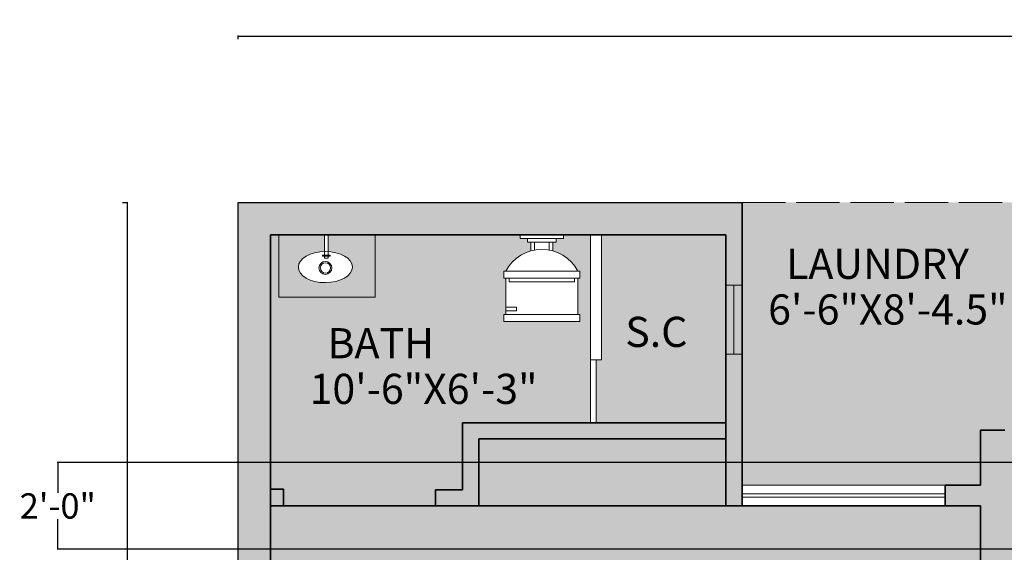
# Model space of a CAD drawing. Units: inches. Extents: x 1884 to 2398, y 474 to 1488.
# Tile 36 of 39: x 1892 to 2165, y 1310 to 1457. Entities that reach past the tile are written whole.
import ezdxf

# ---------------------------------------------------------------- set-up
doc = ezdxf.new("R2010")
doc.units = ezdxf.units.IN
doc.header["$MEASUREMENT"] = 0
doc.linetypes.add('ACAD_ISO02W100', pattern=[15, 12, -3])
doc.layers.get('0').update_dxf_attribs({"color": 250})
for name, color, linetype, lineweight in [('A-ANNO-DIMS', 2, 'Continuous', 18), ('A-AREA-IDEN', 7, 'Continuous', 18), ('A-FLOR-CASE', 8, 'Continuous', 20), ('A-FLOR-FIXT', 8, 'Continuous', 18), ('A-FLOR-OVHD', 8, 'ACAD_ISO02W100', 18), ('A-FLOR-PATT', 254, 'Continuous', 13), ('A-WALL-PATT', 250, 'Continuous', 13), ('C-PROP', 7, 'Continuous', 30), ('walls', 7, 'Continuous', 35), ('windows', 4, 'Continuous', 18)]:
    doc.layers.add(name, color=color, linetype=linetype, lineweight=lineweight)
doc.layers.add('A-FLOR-CASE-PATT', color=251, linetype='Continuous', lineweight=13, true_color=0x636466)
doc.styles.get("Standard").update_dxf_attribs({"font": 'arial.ttf'})
doc.dimstyles.get("Standard").update_dxf_attribs({"dimtxt": 7, "dimasz": 0.18, "dimexe": 0.18, "dimexo": 0.0625, "dimgap": 0.09, "dimtad": 0, "dimtih": 1, "dimtoh": 1, "dimzin": 0, "dimdsep": 46, "dimlunit": 3, "dimtxsty": 'Standard', "dimcen": 0.09, "dimadec": 0, "dimazin": 0, "dimtfac": 1, "dimtofl": 0, "dimtmove": 0, "dimatfit": 3, "dimfxl": 1, "dimtolj": 1, "dimtzin": 0, "dimarcsym": 0})

# ---------------------------------------------------------------- blocks, each defined once
blk = doc.blocks.new('*D1')
at = {"layer": 'A-ANNO-DIMS', "color": 0, "lineweight": -2, "transparency": 16777216}
for p, q in [((1952.529060307534, 1452.046209673956), (1952.529060307534, 1453.03337366088)), ((1952.709060307533, 1452.85337366088), (2168.501475041503, 1452.85337366088)), ((2396.349060307533, 1452.85337366088), (2180.556645573564, 1452.85337366088)), ((2396.529060307533, 1452.046209673956), (2396.529060307533, 1453.03337366088))]:
    blk.add_line(p, q, dxfattribs=at)
at = {"layer": 'A-ANNO-DIMS', "color": 0, "lineweight": 100, "transparency": 16777216}
for points in [[(1952.709060307533, 1452.88337366088), (1952.709060307533, 1452.823373660879), (1952.529060307534, 1452.85337366088)], [(2396.349060307533, 1452.88337366088), (2396.349060307533, 1452.823373660879), (2396.529060307533, 1452.85337366088)]]:
    blk.add_solid(points, dxfattribs=at)
at = {"layer": 'Defpoints', "color": 0, "lineweight": 100, "transparency": 16777216}
for p in [(2396.529060307533, 1452.85337366088), (1952.529060307534, 1451.983709673957), (2396.529060307533, 1451.983709673956)]:
    blk.add_point(p, dxfattribs=at)
at = {"layer": 'A-ANNO-DIMS', "color": 0, "transparency": 16777216, "insert": (2174.529060307534, 1452.85337366088), "char_height": 7, "attachment_point": 5}
blk.add_mtext("\\A1;37'", dxfattribs=at)
blk = doc.blocks.new('*D2')
at = {"layer": 'A-ANNO-DIMS', "color": 0, "lineweight": -2, "transparency": 16777216}
for p, q in [((1920.507592151937, 1406.884736586432), (1921.961917670096, 1406.884736586432)), ((1921.781917670096, 1406.704736586432), (1921.781917670096, 972.551134949324)), ((1921.781917670096, 531.0647365864316), (1921.781917670096, 965.2183382235396)), ((1920.507592151937, 530.8847365864316), (1921.961917670096, 530.8847365864316))]:
    blk.add_line(p, q, dxfattribs=at)
at = {"layer": 'A-ANNO-DIMS', "color": 0, "lineweight": 100, "transparency": 16777216}
for points in [[(1921.751917670096, 1406.704736586432), (1921.811917670096, 1406.704736586432), (1921.781917670096, 1406.884736586432)], [(1921.751917670096, 531.0647365864316), (1921.811917670096, 531.0647365864316), (1921.781917670096, 530.8847365864316)]]:
    blk.add_solid(points, dxfattribs=at)
at = {"layer": 'Defpoints', "color": 0, "lineweight": 100, "transparency": 16777216}
for p in [(1920.445092151936, 1406.884736586432), (1920.445092151937, 530.8847365864316), (1921.781917670096, 530.8847365864316)]:
    blk.add_point(p, dxfattribs=at)
at = {"layer": 'A-ANNO-DIMS', "color": 0, "transparency": 16777216, "insert": (1921.781917670095, 968.884736586431), "char_height": 7, "attachment_point": 5}
blk.add_mtext("\\A1;73'", dxfattribs=at)
blk = doc.blocks.new('*U9')
for p, q in [((-10, 22), (-10, 12)), ((10, 12), (10, 22)), ((-10, 21), (-7, 21)), ((-7, 20), (-10, 20)), ((-7, 21), (-7, 20)), ((10.5, 12), (-10.5, 12)), ((-10.5, 10), (-10.5, 12)), ((9, 13), (-9, 13)), ((-9, 13), (-9, 12)), ((9, 12), (9, 13)), ((10.5, 12), (10.5, 10)), ((10.5, 10), (-10.5, 10)), ((-3, 4.406499999999937), (-3, 2)), ((-2, 2), (-2, 4.16579999999999)), ((2, 4.16579999999999), (2, 2)), ((3, 2), (3, 4.406499999999937)), ((4, 2), (-4, 2)), ((-4, 2), (-4, 1)), ((4, 1), (4, 2))]:
    blk.add_line(p, q)
for points in [[(10.5, 22), (10.5, 24), (-10.5, 24), (-10.5, 22)], [(6, 0), (6, 1), (-6, 1), (-6, 0)]]:
    blk.add_lwpolyline(points, close=True)
blk.add_arc((0, 15.33330000000001), 11.33333, 208.0725, 331.9275)
blk = doc.blocks.new('LAV-OVAL-WITH-TAP')
for p, q in [((7.274409562516666, 6.788668499560117), (7.274409562516666, 13.20873658643177)), ((8.219307397775992, 6.788668499560117), (8.219307397775992, 13.20873658643177)), ((6.697205447740998, 7.581094872117319), (8.82130564205363, 7.581094872117319)), ((6.69720544774077, 7.285663748863044), (6.697205447740998, 7.581094872117319)), ((8.82130564205363, 7.285663748863044), (6.69720544774077, 7.285663748863044)), ((7.274409562516666, 6.788668499560117), (8.219307397775992, 6.788668499560117)), ((8.82130564205363, 7.581094872117319), (8.82130564205363, 7.285663748863044))]:
    blk.add_line(p, q)
for radius in [1.786721855987963, 1.786721855987973, 1.426627914243592, 1.426627914243628, 1.42662769250472, 1.426627377330596]:
    blk.add_circle((7.497021151795252, 4.073758747890906), radius)
blk.add_ellipse((7.480663978300754, 4.312467997805015), major_axis=(-7.480193534640648, -0.0164125256646912), ratio=0.5765346257282574)
blk = doc.blocks.new('*D46')
at = {"layer": 'A-ANNO-DIMS', "color": 0, "lineweight": -2, "transparency": 16777216}
for p, q in [((2247.054069000001, 1334.884737), (1902.431692000002, 1334.884737)), ((1902.611692000002, 1334.704737), (1902.611692000002, 1326.548747914052)), ((1902.611692000002, 1311.064737), (1902.611692000002, 1319.220726085948)), ((2242.554069000001, 1310.884737), (1902.431692000002, 1310.884737))]:
    blk.add_line(p, q, dxfattribs=at)
at = {"layer": 'A-ANNO-DIMS', "color": 0, "lineweight": 100, "transparency": 16777216}
for points in [[(1902.581692000002, 1334.704737), (1902.641692000002, 1334.704737), (1902.611692000002, 1334.884737)], [(1902.581692000002, 1311.064737), (1902.641692000002, 1311.064737), (1902.611692000002, 1310.884737)]]:
    blk.add_solid(points, dxfattribs=at)
at = {"layer": 'Defpoints', "color": 0, "lineweight": 100, "transparency": 16777216}
for p in [(2247.116569000001, 1334.884737), (1902.611692000002, 1310.884737), (2242.616569000001, 1310.884737)]:
    blk.add_point(p, dxfattribs=at)
at = {"layer": 'A-ANNO-DIMS', "color": 0, "transparency": 16777216, "insert": (1902.611692000002, 1322.884737), "char_height": 7, "attachment_point": 5}
blk.add_mtext('\\A1;2\'-0"', dxfattribs=at)

msp = doc.modelspace()

# ---------------------------------------------------------------- hatches: boundary and pattern name
at = {"layer": 'A-FLOR-CASE-PATT'}
h = msp.add_hatch(color=256, dxfattribs=at)
h.dxf.hatch_style = 1
edge = h.paths.add_edge_path()
edge.add_line((1976.467409562516, 1397.884736586431), (1963.77207706678, 1397.884736586431))
edge.add_line((1963.77207706678, 1397.884736586431), (1963.77207706678, 1380.629613732504))
edge.add_line((1963.77207706678, 1380.629613732504), (1990.418484078909, 1380.629613732504))
edge.add_line((1990.418484078909, 1380.629613732504), (1990.41848407891, 1397.884736586431))
edge.add_line((1990.41848407891, 1397.884736586431), (1977.412307397776, 1397.884736586431))
edge.add_line((1977.412307397776, 1397.884736586431), (1977.412307397776, 1393.281080523333))
edge.add_ellipse((1976.673663978301, 1388.988467997805), major_axis=(-7.480193534640648, -0.0164125256646912), ratio=0.5765346257282575, start_angle=272.6136539907866, end_angle=620.1108329880406, ccw=False)
edge.add_line((1976.467409562516, 1393.299134032605), (1976.467409562516, 1397.884736586431))
h = msp.add_hatch(color=256, dxfattribs=at)
h.dxf.hatch_style = 1
h.paths.add_polyline_path([(2230.029060307534, 1334.884736586432), (2167.029060307534, 1334.884736586432), (2167.029060307533, 1252.384736586432), (2188.39223788629, 1252.384736586432), (2188.39223788629, 1308.548092360888), (2230.029060307534, 1308.548092360888)])
h.paths.add_polyline_path([(2087.529060307534, 1341.419208402589), (2019.112052587603, 1341.419208402589), (2019.112052587603, 1327.384736586431), (2019.112052587603, 1322.884736586432), (2087.529060307534, 1322.884736586431)])
at = {"layer": 'A-FLOR-PATT'}
h = msp.add_hatch(color=256, dxfattribs=at)
h.dxf.hatch_style = 1
h.paths.add_polyline_path([(2170.029060307534, 1403.884736586431), (2170.029060307534, 1406.884736586431), (2092.029060307534, 1406.884736586431), (2092.029060307534, 1328.62308547235), (2148.233210584229, 1328.62308547235), (2158.029060307534, 1328.62308547235), (2158.029060307534, 1334.884736586432), (2158.029060307534, 1343.884736586432), (2164.725919940865, 1343.884736586432), (2170.029060307534, 1343.884736586432)])
h = msp.add_hatch(color=256, dxfattribs=at)
h.dxf.hatch_style = 1
h.paths.add_polyline_path([(2050.106778681225, 1363.349576779681), (2050.106778681225, 1397.884736586431), (2042.590228763987, 1397.884736586431), (2042.590228763987, 1396.884736586432), (2040.590228763988, 1396.884736586432), (2040.590228763988, 1395.884736586431), (2039.590228763987, 1395.884736586431), (2039.590228763987, 1393.480497336967, -0.2060810176159205), (2046.590242763922, 1387.884736586431), (2047.090228763988, 1387.884736586431), (2047.090228763988, 1385.884736586431), (2046.590228763987, 1385.884736586431), (2046.590228763987, 1375.884736586432), (2047.090228763988, 1375.884736586432), (2047.090228763988, 1373.884736586431), (2026.090228763988, 1373.884736586431), (2026.090228763988, 1375.884736586432), (2026.590228763987, 1375.884736586432), (2026.590228763987, 1385.884736586431), (2026.090228763988, 1385.884736586431), (2026.090228763988, 1387.884736586431), (2026.590214764052, 1387.884736586431, -0.2060810176159205), (2033.590228763987, 1393.480497336967), (2033.590228763987, 1395.884736586431), (2032.590228763988, 1395.884736586431), (2032.590228763988, 1396.884736586432), (2030.590228763987, 1396.884736586432), (2030.590228763987, 1397.884736586431), (1990.41848407891, 1397.884736586431), (1990.418484078909, 1380.629613732504), (1963.77207706678, 1380.629613732504), (1963.77207706678, 1397.884736586431), (1961.529060307533, 1397.884736586431), (1961.529060307533, 1327.560779427295), (1965.065804798096, 1327.560779427295), (1965.065804798096, 1322.884736586432), (2007.131770728449, 1322.884736586432), (2007.131770728449, 1327.384736586431), (2014.612052587603, 1327.384736586431), (2014.612052587603, 1345.919208402589), (2050.106778681225, 1345.919208402589)])
h.paths.add_polyline_path([(2087.529060307534, 1397.884736586431), (2053.062200912405, 1397.884736586431), (2053.062200912405, 1363.349576779681), (2051.584489796816, 1363.349576779681), (2051.584489796816, 1345.919208402589), (2087.529060307534, 1345.919208402589)])
h.paths.add_polyline_path([(2301.255122477188, 1334.884736586432), (2265.892029109202, 1334.884736586432), (2259.116568963785, 1334.884736586432), (2259.116568963785, 1333.884736586432), (2257.116568963786, 1333.884736586432), (2257.116568963786, 1332.884736586432), (2256.116568963786, 1332.884736586432), (2256.116568963786, 1330.480497336967, -0.2060810176159197), (2263.116582963721, 1324.884736586432), (2263.616568963786, 1324.884736586432), (2263.616568963786, 1322.884736586432), (2263.116568963786, 1322.884736586432), (2263.116568963786, 1312.884736586432), (2263.616568963786, 1312.884736586432), (2263.616568963786, 1310.884736586432), (2242.616568963786, 1310.884736586432), (2242.616568963786, 1312.884736586432), (2243.116568963785, 1312.884736586432), (2243.116568963785, 1322.884736586432), (2242.616568963786, 1322.884736586432), (2242.616568963786, 1324.884736586432), (2243.11655496385, 1324.884736586432, -0.2060810176159197), (2250.116568963786, 1330.480497336967), (2250.116568963786, 1332.884736586432), (2249.116568963786, 1332.884736586432), (2249.116568963786, 1333.884736586432), (2247.116568963786, 1333.884736586432), (2247.116568963786, 1334.884736586432), (2234.529060307534, 1334.884736586432), (2234.529060307533, 1275.553826810391), (2230.029060307533, 1275.553826810391), (2230.029060307533, 1256.117249027531), (2234.529060307533, 1256.117249027531), (2234.529060307533, 1252.384736586432), (2265.892029109202, 1252.384736586432), (2301.255122477188, 1252.384736586432)])
h.paths.add_polyline_path([(2283.754419727821, 1281.541714860787), (2301.009542581749, 1281.541714860787), (2301.009542581749, 1254.895307848658), (2283.754419727821, 1254.895307848658)], flags=16)
edge = h.paths.add_edge_path(flags=0)
edge.add_ellipse((2292.113273993122, 1268.640127949267), major_axis=(-0.0164125256646898, 7.480193534640649), ratio=0.5765346257282574, start_angle=272.6136539907895, end_angle=620.1108329880437, ccw=False)
edge.add_ellipse((2292.113273993122, 1268.640127949267), major_axis=(-0.0164125256646898, 7.480193534640649), ratio=0.5765346257282574, start_angle=260.1108329880437, end_angle=272.6136539907895, ccw=False)
h.paths.add_polyline_path([(2293.661286599196, 1268.623770775773, -1), (2290.08784288722, 1268.623770775773, -1)], flags=0)
h.paths.add_polyline_path([(2290.447937365877, 1268.623770775773, -1), (2293.301192120539, 1268.623770775773, -1)], flags=0)
h.paths.add_polyline_path([(2295.08646974418, 1269.423586479827), (2295.381900867434, 1269.423586479827), (2295.381900867434, 1267.299486285514), (2295.08646974418, 1267.299486285514), (2295.08646974418, 1267.901484529792), (2294.589474494877, 1267.901484529792), (2294.589474494877, 1268.846382365051), (2295.08646974418, 1268.846382365051)], flags=0)
h.paths.add_polyline_path([(2342.529060307533, 1334.884736586432), (2302.732833592778, 1334.884736586432), (2302.732833592777, 1317.822173990474), (2304.210544708368, 1317.822173990474), (2304.210544708368, 1252.384736586432), (2342.529060307533, 1252.384736586432), (2342.529060307533, 1276.19700522134)])
h = msp.add_hatch(color=256, dxfattribs=at)
h.dxf.hatch_style = 1
h.paths.add_polyline_path([(2117.529060307534, 815.8008601642414), (2126.529060307533, 815.8008601642414), (2126.529060307534, 880.3823245284138), (2117.529060307534, 880.3823245284138), (2117.529060307534, 892.3847365864315), (1961.529060307533, 892.3847365864318), (1961.529060307533, 756.9152132436575), (1964.529060307533, 756.9152132436575), (1964.529060307533, 759.9152132436574), (1995.529060307533, 759.9152132436574), (1995.529060307533, 753.9152132436575), (1972.862393640866, 753.9152132436575), (1967.529060307533, 756.9152132436575), (1967.529060307533, 654.9152132436574), (1972.862393640866, 657.9152132436575), (1995.529060307533, 657.9152132436575), (1995.529060307533, 651.9152132436574), (1964.529060307533, 651.9152132436574), (1964.529060307533, 654.9152132436574), (1961.529060307533, 654.9152132436574), (1961.529060307533, 640.3847365864318), (2117.529060307534, 640.3847365864314), (2117.529060307534, 646.5776756488413), (2126.529060307534, 646.5776756488413), (2126.529060307533, 676.1826019380942), (2117.529060307534, 676.1826019380942)])
h.paths.add_polyline_path([(2012.245892997025, 808.9291988189563), (2012.049579081969, 810.1854570579605), (2032.542313208683, 810.1854570579605), (2032.346024821094, 808.9291988189563)], flags=16)
h.paths.add_polyline_path([(2010.38119353609, 820.8636520894975), (1994.658277650963, 820.8636520894975), (1994.658277650963, 831.5614635913172), (1984.608211738929, 833.1317793251212), (1984.608211738929, 853.8208002572304), (1994.658277650963, 855.3911120678468), (1994.658277650963, 866.0889486936543), (2010.381193536673, 866.0889486936543), (2011.951435886253, 876.1390146056889), (2032.640472118199, 876.1390146056889), (2034.210849866988, 866.0889486936543), (2045.556424228796, 866.0889486936543), (2047.126666578375, 876.1390146056889), (2067.815702810321, 876.1390146056889), (2069.386080559109, 866.0889486936543), (2085.108870859277, 866.0889486936543), (2085.108870859277, 855.3911120678468), (2095.158936771312, 853.8208002572304), (2095.158936771312, 833.1317793251212), (2085.108870859277, 831.5614635913172), (2085.108870859277, 820.8636520894975), (2069.386080560277, 820.8636520894975), (2067.815706736618, 810.8135861774629), (2047.126664615719, 810.8135861774629), (2045.556424228212, 820.8636520894975), (2034.210849868156, 820.8636520894975), (2032.640476044496, 810.8135861774629), (2011.951433923597, 810.8135861774629)], flags=16)
h.paths.add_polyline_path([(1982.723824380422, 833.426234479541), (1982.723824380422, 853.5263663036108), (1983.980082619426, 853.7226346601389), (1983.980082619426, 833.2299276462522)], flags=16)
h.paths.add_polyline_path([(1994.529060307533, 753.5402132436574), (1994.529060307533, 658.2902132436575), (1973.529060307533, 658.2902132436575), (1973.529060307533, 753.5402132436574)], flags=16)
h.paths.add_polyline_path([(2084.48576677273, 843.5274175393209), (2084.59204621975, 843.5024682506945), (2084.680989303072, 843.4873429014967), (2084.812983397052, 843.4769081193547), (2084.91314582564, 843.4767023942125), (2084.66880953484, 843.4819332556493), (2084.336020790642, 843.5646279083602), (2084.11630122464, 843.6165616239609), (2083.80035227753, 843.6856683896884), (2083.105016757222, 843.8265189249884), (2082.836048453269, 843.873780498397), (2083.603851506107, 843.7286485385392), (2084.20582336258, 843.5969806585211)], flags=0)
h.paths.add_polyline_path([(2047.421123689146, 808.9291988189563), (2047.224809774091, 810.1854570579605), (2067.717543900804, 810.1854570579605), (2067.521255513216, 808.9291988189563)], flags=16)
h.paths.add_polyline_path([(2066.009851225869, 849.5050711179754), (2066.42856209693, 849.6872536877958), (2066.798278896669, 849.8816973380289), (2067.128674813528, 850.0847337946167), (2067.429674287593, 850.2926822209193), (2067.71107613313, 850.501861780296), (2068.176225202245, 850.8560509488422), (2068.688503010997, 851.2051162670248), (2069.305475594623, 851.5305287965867), (2070.015309134756, 851.783837036287), (2070.843781436505, 851.9440833228273), (2071.080737607611, 851.9560435048553), (2070.628610267393, 851.9024640909616), (2070.212160661163, 851.8219128126768), (2069.82749438838, 851.7168142484016), (2069.471093925975, 851.5896306642849), (2069.13919049923, 851.4428243264747), (2068.828266585076, 851.2788323759551), (2068.534427782973, 851.1001296414569), (2068.254156569851, 850.9091532639633), (2067.982553538579, 850.708579073524), (2067.501844470646, 850.3425416967154), (2066.951193479014, 849.9621190813364), (2066.223646961128, 849.579483505263)], flags=0)
h.paths.add_polyline_path([(2059.423038027123, 853.2214975541691), (2059.826673799315, 853.277727672947), (2060.171391060097, 853.3584925151328), (2060.464601733081, 853.462573510234), (2060.713717741875, 853.5887269625948), (2060.925899758443, 853.7357343017233), (2061.107303448155, 853.9021759558088), (2061.257928811012, 854.0857906600216), (2061.376770840422, 854.2841287107957), (2061.462447652322, 854.4947278419824), (2061.513828614297, 854.7151509125981), (2061.529531842285, 854.9429230939121), (2061.508426703869, 855.1756072449404), (2061.449382566637, 855.4107536621171), (2061.352399430585, 855.6463020819306), (2061.223632961088, 855.8818505017439), (2061.070243830105, 856.1173989215573), (2060.899769587072, 856.3529473413709), (2060.719370903951, 856.588495761183), (2060.405833605864, 856.9925386710904), (2060.102852609014, 857.4235624716171), (2059.858108421559, 857.8880530440814), (2059.691164532255, 858.4673451479222), (2059.835525259983, 859.0912752050886), (2060.304837982534, 859.5324417717479), (2060.843952795028, 859.7984964546366), (2061.512696715463, 859.9353091544514), (2062.253367096678, 859.9051905068), (2062.482906219865, 859.8492647715083), (2062.077511686138, 859.9123414976887), (2061.695357929833, 859.9278814121051), (2061.33644495095, 859.8992512868383), (2061.004667150029, 859.8313756541849), (2060.703416424316, 859.7291413586948), (2060.436587174351, 859.5974603700822), (2060.207822549028, 859.4412446580619), (2060.020765697241, 859.2654061923486), (2059.879059767881, 859.0748318174917), (2059.785217277427, 858.8738430618334), (2059.736725709402, 858.6642614998202), (2059.729941914911, 858.4473182645266), (2059.761222745062, 858.2242444890267), (2059.826925050962, 857.9962587438123), (2059.92315443207, 857.7646047245396), (2060.04651899114, 857.5304758765365), (2060.193124327632, 857.2951410206236), (2060.358699163532, 857.0595926008104), (2060.536585330176, 856.8240441809971), (2060.866718458323, 856.3986148921463), (2061.170885250692, 855.9783402158826), (2061.422381845951, 855.5182854684566), (2061.56688892396, 854.942778343735), (2061.410468633091, 854.271739120365), (2060.947138393936, 853.7069322166539), (2060.334567557683, 853.3967236267573), (2059.649288497294, 853.2361675378636)], flags=0)
h.paths.add_polyline_path([(2050.777720077942, 859.7454978409666), (2051.07042824763, 859.870219158935), (2051.294544717468, 860.017025496745), (2051.46690334786, 860.1832661495123), (2051.593911055823, 860.3654487193328), (2051.679210990252, 860.5598923695659), (2051.726446300039, 860.7629288261536), (2051.739260134076, 860.9708772524561), (2051.721546892906, 861.1800568118329), (2051.676698473774, 861.386774105061), (2051.60860927722, 861.5873482955004), (2051.521299329609, 861.7789402395308), (2051.420547418841, 861.9619393772065), (2051.312383584462, 862.1375768416017), (2051.202963491846, 862.3070837657913), (2050.966442536983, 862.6795474136981), (2050.793480878491, 863.1925713661464), (2051.021372914674, 863.6992722615545), (2051.482558609153, 864.0178750295152), (2052.090482216228, 864.1376203451599), (2052.773111098533, 864.157049396074), (2053.006824697232, 864.1424016774818), (2052.60318892504, 864.1522130543284), (2052.258471664257, 864.1424016774818), (2051.965260991273, 864.1129549843595), (2051.716144982478, 864.063885537544), (2051.50396296591, 863.9951807744528), (2051.322433650375, 863.907255260305), (2051.170300777631, 863.8021566960299), (2051.04756434768, 863.6823473477759), (2050.954349986346, 863.5502517939447), (2050.890532067805, 863.4083574258491), (2050.85623621788, 863.2590888218906), (2050.851336810748, 863.1049208108001), (2050.875833846408, 862.9483030961434), (2050.928847944094, 862.7910572523672), (2051.005102819202, 862.6326054006817), (2051.09844280636, 862.4716787202652), (2051.202963491844, 862.3070837657904), (2051.312383584462, 862.1375768416013), (2051.556251316974, 861.7415820950013), (2051.751339156135, 861.1669008329959), (2051.712429226858, 860.5354537160036), (2051.398466566313, 860.0850989679107), (2050.948595340801, 859.7904131416026)], flags=0)
h.paths.add_polyline_path([(2022.768265091874, 719.2635269564156), (2050.460701888225, 719.2635269564156), (2050.460701888225, 717.2264308545614), (2052.426027545829, 717.2264308545614), (2052.426027545829, 715.0328555474166), (2050.460701888225, 715.0328555474166), (2050.460701888225, 703.7384712949378), (2022.768265091874, 703.7384712949378)], flags=16)
h.paths.add_polyline_path([(2012.245892997025, 878.0234019641955), (2032.346024821094, 878.0234019641955), (2032.542311246466, 876.7671437251912), (2012.049583009897, 876.7671437251912)], flags=16)
h.paths.add_polyline_path([(2035.324314229629, 713.1026297220419), (2035.342323734454, 713.2939269647811), (2035.191594480285, 713.2022463391573)], flags=0)
h.paths.add_polyline_path([(2036.483793368253, 711.6303552235653), (2036.583057308503, 711.849035191806), (2036.389574164252, 711.8976249102717)], flags=0)
h.paths.add_polyline_path([(2036.073963013272, 712.7444251806157), (2035.992966259493, 712.4813789411762), (2035.723718538195, 712.5164991793641), (2035.794480886751, 712.7255350820222)], flags=0)
h.paths.add_polyline_path([(2035.845889740907, 710.9094011156075), (2035.752657170415, 710.9579395480923), (2035.701796841489, 710.8802910191051)], flags=0)
h.paths.add_polyline_path([(2037.817833105062, 712.0186444527698), (2037.94771907015, 712.060054181353), (2037.986590761345, 712.1613470938162), (2037.815493232997, 712.0195830652098)], flags=0)
h.paths.add_polyline_path([(2038.451438253888, 709.5174527548473), (2038.46381259532, 709.4275335183239), (2038.585708407037, 709.4415430414689)], flags=0)
h.paths.add_polyline_path([(2037.805223875722, 709.8056815263456), (2037.818420097464, 709.807253189157), (2037.804492020793, 709.8227772356641)], flags=0)
h.paths.add_polyline_path([(2036.699670737428, 711.2453724121245), (2036.698482732612, 711.2358968812113), (2036.813156202547, 711.2113760065187)], flags=0)
h.paths.add_polyline_path([(2035.92842163957, 708.8974795736603), (2035.668252200497, 708.8712447892582), (2035.705968573039, 708.6672524113528)], flags=0)
h.paths.add_polyline_path([(2036.4135388155, 710.9761633445361), (2035.932343572741, 709.8585852823189), (2036.792006299979, 710.4843975690396), (2036.499859551577, 710.934168748562)], flags=0)
h.paths.add_polyline_path([(2038.297960372458, 712.1148420018311), (2038.498945749665, 712.0579037604177), (2038.612442111864, 712.268650843707), (2038.390256576993, 712.3323300722286)], flags=0)
h.paths.add_polyline_path([(2047.421123689146, 878.0234019641955), (2067.521255513216, 878.0234019641955), (2067.717541938588, 876.7671437251912), (2047.224813702019, 876.7671437251912)], flags=16)
h.paths.add_polyline_path([(2049.647427742059, 705.0928292249858, -1), (2048.84548899896, 705.0928292249858, -1)], flags=0)
h.paths.add_polyline_path([(2095.787065890814, 853.7226542967927), (2097.043324129819, 853.5263663036108), (2097.043324129819, 833.426234479541), (2095.787065890814, 833.2299276462522)], flags=16)
h.paths.add_polyline_path([(2110.738728909887, 745.3388006828269), (2111.750023094465, 745.3388006828269, -0.0640418572917222), (2113.266964371214, 742.919542441155), (2113.266964371214, 732.1919762839284), (2113.525533380085, 732.1919762839282, -0.4142135623731062), (2114.278258555744, 731.4392511082686), (2114.278258555744, 716.7639945070974, -0.4142135623730951), (2113.525533380085, 716.0112693314378), (2113.266964371214, 716.0112693314377), (2113.266964371214, 705.2837031743313, -0.0640418572952104), (2111.750023094367, 702.8644449325391), (2110.738728909887, 702.8644449325391), (2110.738728909887, 716.0112693314377), (2109.468865716485, 716.0112693314378, -0.4142135623730951), (2108.716140540826, 716.7639945070974), (2108.716140540826, 731.4392511082686, -0.4142135623730951), (2109.468865716485, 732.1919762839282), (2110.738728909887, 732.1919762839284)], flags=16)
h.paths.add_polyline_path([(1998.045441111793, 668.9094387650339), (2002.449119404415, 668.9094387650339), (2002.449119404415, 652.2733207706847), (2002.724349297704, 652.762618358754), (2002.724349297704, 668.1754923829302), (2019.972089277139, 668.1754923829302), (2019.972089277139, 652.762618358754), (2020.247319170428, 652.2733207706847), (2020.247319170428, 668.9094387650339), (2024.65099746305, 668.9094387650339), (2029.054675755671, 668.9094387650334), (2029.054675755671, 652.2733207706846), (2029.329905648959, 652.7626183587535), (2029.32990564896, 668.1754923829299), (2046.577645628395, 668.1754923829296), (2046.577645628395, 652.7626183587535), (2046.852875521684, 652.2733207706846), (2046.852875521684, 668.9094387650333), (2051.256553814306, 668.9094387650332), (2051.256553814305, 646.1571009198206), (2049.054714667995, 646.1571009198207), (2049.054714667995, 643.9552617735098), (2026.85283660936, 643.9552617735101), (2026.85283660936, 646.157100919821), (2024.650997463049, 646.157100919821), (2022.449158316739, 646.1571009198213), (2022.449158316739, 643.9552617735103), (2000.247280258104, 643.9552617735103), (2000.247280258104, 646.1571009198213), (1998.045441111793, 646.1571009198213)], flags=16)
h.paths.add_polyline_path([(2342.529060307532, 1247.884736586432), (2265.892029109202, 1247.884736586432), (2230.029060307533, 1247.884736586432), (2209.755415465046, 1247.884736586432), (2168.600168546053, 1247.884736586432), (2168.600168546053, 1104.929335189726), (2158.029060307534, 1104.929335189726), (2158.029060307534, 1079.411493140081), (2168.600168546053, 1079.411493140081), (2168.600168546053, 1062.466054843048), (2342.529060307534, 1062.466054843048), (2342.529060307535, 1093.80946809509)])
h.paths.add_polyline_path([(2215.029585767078, 1153.875922220359), (2215.029585767078, 1164.738901046202), (2187.558514037159, 1164.738901046202), (2187.441848177233, 1152.640560104242), (2173.567560328407, 1152.640560104242), (2173.684226188333, 1164.738901046178), (2173.684226188333, 1218.738896358896), (2173.80089204826, 1230.837237300835), (2187.675179897085, 1230.837237300835), (2187.558514037159, 1218.738896358897), (2215.029585767078, 1218.738896358897), (2215.029585767078, 1225.878851812398), (2245.053154048409, 1225.878851812398), (2245.053154048409, 1153.875922220359)], flags=16)
h.paths.add_polyline_path([(2192.146797479106, 1164.797089366358), (2184.963183514796, 1174.540018628516), (2184.914853464182, 1174.540018628516), (2176.755013122293, 1174.540018628516), (2176.755013122293, 1190.362773833876), (2184.914853464182, 1190.362773833876), (2184.914853464182, 1196.818536437712), (2176.755013122293, 1196.818536437712), (2176.755013122293, 1212.641291643072), (2184.914853464182, 1212.641291643072), (2184.914853464182, 1174.605567287827), (2184.963183514796, 1174.540018628516), (2192.146797479106, 1174.540018628516)], flags=0)
h.paths.add_polyline_path([(2184.970820652961, 1158.363900966234, -1), (2176.038587852678, 1158.363900966234, -1)], flags=0)
h.paths.add_polyline_path([(2335.555222872957, 1161.985357442079), (2335.555222872957, 1175.132181840978), (2334.285359679555, 1175.132181840978, -0.4142135623730951), (2333.532634503896, 1175.884907016637), (2333.532634503896, 1190.560163617809, -0.4142135623730951), (2334.285359679555, 1191.312888793468), (2335.555222872957, 1191.312888793468), (2335.555222872957, 1204.459713192367), (2336.566517057534, 1204.459713192367, -0.0640418572917234), (2338.083458334283, 1202.040454950695), (2338.083458334283, 1191.312888793468), (2338.342027343154, 1191.312888793468, -0.4142135623731616), (2339.094752518814, 1190.560163617809), (2339.094752518814, 1175.884907016637, -0.4142135623730951), (2338.342027343154, 1175.132181840978), (2338.083458334283, 1175.132181840978), (2338.083458334283, 1164.404615683871, -0.0640418572952083), (2336.566517057436, 1161.985357442079)], flags=16)
h.paths.add_polyline_path([(2176.155253712605, 1224.462237220889, -1), (2185.087486512887, 1224.462237220889, -1)], flags=0)
h.paths.add_polyline_path([(2158.029060307534, 1276.19700522134), (2158.029060307534, 1322.884736586431), (2148.233210584229, 1322.884736586431), (2092.029060307534, 1322.884736586431), (1961.529060307533, 1322.884736586432), (1961.529060307533, 1166.884736586432), (2116.004926061792, 1166.884736586431), (2116.004926061792, 1157.884736586431), (2152.637676873365, 1157.884736586431), (2152.637676873365, 1166.884736586431), (2158.029060307534, 1166.884736586431)])
h.paths.add_polyline_path([(2006.351794059088, 1204.245313711267), (2006.351794059088, 1215.108292537111), (1978.880722329168, 1215.108292537111), (1978.764056469242, 1203.00995159515), (1964.889768620417, 1203.00995159515), (1965.006434480343, 1215.108292537088), (1965.006434480343, 1269.108287849805), (1965.123100340269, 1281.206628791743), (1978.997388189094, 1281.206628791743), (1978.880722329168, 1269.108287849805), (2006.351794059088, 1269.108287849805), (2006.351794059088, 1276.248243303306), (2036.375362340419, 1276.248243303306), (2036.375362340419, 1204.245313711267)], flags=16)
h.paths.add_polyline_path([(1983.469005771116, 1215.166480857267), (1976.285391806805, 1224.909410119424), (1976.237061756191, 1224.909410119424), (1968.077221414302, 1224.909410119424), (1968.077221414302, 1240.732165324784), (1976.237061756191, 1240.732165324784), (1976.237061756191, 1247.18792792862), (1968.077221414302, 1247.18792792862), (1968.077221414302, 1263.01068313398), (1976.237061756191, 1263.01068313398), (1976.237061756191, 1224.974958778736), (1976.285391806805, 1224.909410119424), (1983.469005771116, 1224.909410119424)], flags=0)
h.paths.add_polyline_path([(1976.293028944971, 1208.733292457142, -1), (1967.360796144688, 1208.733292457142, -1)], flags=0)
h.paths.add_polyline_path([(1967.477462004614, 1274.831628711797, -1), (1976.409694804897, 1274.831628711797, -1)], flags=0)
h.paths.add_polyline_path([(2152.586710801799, 1223.485042164994), (2152.586710801799, 1236.631866563892), (2151.316847608397, 1236.631866563892, -0.4142135623730951), (2150.564122432737, 1237.384591739552), (2150.564122432737, 1252.059848340723, -0.4142135623730951), (2151.316847608397, 1252.812573516383), (2152.586710801799, 1252.812573516383), (2152.586710801799, 1265.959397915281), (2153.598004986376, 1265.959397915281, -0.0640418572917215), (2155.114946263125, 1263.54013967361), (2155.114946263125, 1252.812573516383), (2155.373515271996, 1252.812573516383, -0.4142135623730288), (2156.126240447656, 1252.059848340723), (2156.126240447656, 1237.384591739552, -0.4142135623730951), (2155.373515271996, 1236.631866563892), (2155.114946263125, 1236.631866563892), (2155.114946263125, 1225.904300406786, -0.0640418572952094), (2153.598004986278, 1223.485042164994)], flags=16)
h.paths.add_polyline_path([(2250.676094667158, 1161.100728645635), (2322.077457416915, 1161.100728645635), (2322.077457416915, 1173.885720445675), (2250.676094667158, 1173.885720445675)], flags=24)
h.paths.add_polyline_path([(2255.610417877832, 1173.711980483038), (2320.135651303891, 1173.711980483038), (2320.135651303891, 1186.659131725134), (2255.610417877832, 1186.659131725134)], flags=24)
h.paths.add_polyline_path([(2053.687197260262, 1230.837005449875), (2125.088560010019, 1230.837005449875), (2125.088560010019, 1243.621997249915), (2053.687197260262, 1243.621997249915)], flags=24)
h.paths.add_polyline_path([(2058.621520470935, 1243.448257287277), (2123.146753896995, 1243.448257287277), (2123.146753896995, 1256.395408529374), (2058.621520470935, 1256.395408529374)], flags=24)
at = {"layer": 'A-WALL-PATT'}
h = msp.add_hatch(color=256, dxfattribs=at)
h.dxf.hatch_style = 1
h.paths.add_polyline_path([(2092.029060307534, 1406.884736586431), (1952.529060307534, 1406.884736586431), (1952.529060307534, 939.2494405891929), (1955.529060307533, 939.2494405891929), (1955.529060307534, 1069.384736586431), (1969.694531803689, 1069.384736586431), (1969.694531803689, 1078.384736586431), (1961.529060307533, 1078.384736586431), (1961.529060307533, 1397.884736586431), (2087.529060307534, 1397.884736586431), (2087.529060307534, 1322.884736586431), (2092.029060307534, 1322.884736586431), (2092.029060307534, 1328.62308547235)])
h.paths.add_polyline_path([(2087.529060307534, 1345.919208402589), (2014.612052587603, 1345.919208402589), (2014.612052587603, 1327.384736586431), (2007.131770728449, 1327.384736586431), (2007.131770728449, 1322.884736586432), (2019.112052587603, 1322.884736586432), (2019.112052587603, 1327.384736586431), (2019.112052587603, 1341.419208402589), (2087.529060307534, 1341.419208402589)], flags=17)
h.paths.add_polyline_path([(1965.065804798096, 1327.560779427295), (1961.529060307533, 1327.560779427295), (1961.529060307533, 1322.884736586432), (1965.065804798096, 1322.884736586432)], flags=17)
h.paths.add_polyline_path([(2351.529060307534, 1343.884736586431), (2265.892029109202, 1343.884736586432), (2164.725919940865, 1343.884736586432), (2158.029060307534, 1343.884736586432), (2158.029060307534, 1334.884736586432), (2158.029060307534, 1328.62308547235), (2148.233210584229, 1328.62308547235), (2148.233210584229, 1322.884736586431), (2158.029060307534, 1322.884736586431), (2158.029060307534, 1276.19700522134), (2158.029060307534, 1166.884736586431), (2152.637676873365, 1166.884736586431), (2152.637676873365, 1157.884736586431), (2158.029060307534, 1157.884736586431), (2158.029060307534, 1104.929335189726), (2168.600168546053, 1104.929335189726), (2168.600168546053, 1247.884736586432), (2209.755415465046, 1247.884736586432), (2209.755415465046, 1252.384736586432), (2167.029060307533, 1252.384736586432), (2167.029060307534, 1334.884736586432), (2265.892029109202, 1334.884736586432), (2342.529060307533, 1334.884736586432), (2342.529060307533, 1310.040870903886), (2351.529060307534, 1310.040870903886)])
h.paths.add_polyline_path([(2234.529060307534, 1334.884736586432), (2230.029060307534, 1334.884736586432), (2230.029060307533, 1275.553826810391), (2234.529060307533, 1275.553826810391)], flags=17)
h.paths.add_polyline_path([(2342.529060307533, 1252.384736586432), (2265.892029109202, 1252.384736586432), (2234.529060307533, 1252.384736586432), (2234.529060307533, 1256.117249027531), (2230.029060307533, 1256.117249027531), (2230.029060307533, 1247.884736586432), (2265.892029109202, 1247.884736586432), (2342.529060307533, 1247.884736586432)], flags=17)
h.paths.add_polyline_path([(2351.529060307534, 1276.19700522134), (2351.529060307534, 1293.634736586432), (2342.529060307533, 1293.634736586432), (2342.529060307533, 1252.384736586432), (2342.529060307533, 1225.301741208246), (2346.310886507181, 1225.301741208246), (2351.529060307534, 1225.301741208246)], flags=17)
h.paths.add_polyline_path([(2351.529060307534, 1126.263620407819), (2342.529060307534, 1126.263620407819), (2342.529060307534, 1093.80946809509), (2342.529060307534, 1062.466054843048), (2168.600168546053, 1062.466054843048), (2168.600168546053, 1079.411493140081), (2158.029060307534, 1079.411493140081), (2158.029060307534, 1056.803418329815), (2158.029060307531, 1053.466054843047), (2213.529060307534, 1053.466054843047), (2213.529060307534, 934.6750023260108), (2222.529060307534, 934.6750023260108), (2222.529060307534, 1057.966054843047), (2342.529060307533, 1057.966054843047), (2342.529060307533, 1027.205699385667), (2345.987405996661, 1027.205699385667), (2351.529060307534, 1027.205699385667)])
h.paths.add_polyline_path([(2116.004926061792, 1166.884736586431), (1961.529060307533, 1166.884736586432), (1961.529060307533, 1162.384736586432), (2081.529060307534, 1162.384736586431), (2081.529060307534, 1152.291637361548), (2090.529060307534, 1152.291637361548), (2090.529060307534, 1157.884736586431), (2116.004926061792, 1157.884736586431)])
h.paths.add_polyline_path([(2090.529060307534, 1122.634736586431), (2081.529060307534, 1122.634736586431), (2081.529060307534, 1078.384736586431), (2000.529060307534, 1078.384736586431), (2000.529060307534, 1069.384736586431), (2000.529060307534, 1034.462559733458), (2003.892918808244, 1034.462559733458), (2009.529060307534, 1034.462559733458), (2009.529060307534, 1069.384736586431), (2090.529060307534, 1069.384736586431)], flags=17)
h.paths.add_polyline_path([(2351.529060307534, 974.6759340295412), (2342.529060307533, 974.6759340295412), (2342.529060307533, 951.8600608887581), (2351.529060307534, 951.8600608887581)], flags=17)

# ---------------------------------------------------------------- linework, layer by layer
at = {"layer": 'A-FLOR-CASE'}
for p, q in [((1963.77207706678, 1397.884736586431), (1963.77207706678, 1380.629613732504)), ((1990.418484078909, 1380.629613732504), (1990.41848407891, 1397.884736586431)), ((1963.77207706678, 1380.629613732504), (1990.418484078909, 1380.629613732504))]:
    msp.add_line(p, q, dxfattribs=at)
at = {"layer": 'A-FLOR-FIXT'}
for p, q in [((2050.106778681225, 1397.884736586431), (2050.106778681225, 1363.349576779681)), ((2053.062200912405, 1363.349576779681), (2053.062200912405, 1397.884736586431)), ((2050.106778681225, 1363.349576779681), (2053.062200912405, 1363.349576779681)), ((2050.106778681225, 1363.349576779681), (2050.106778681225, 1345.983839034574)), ((2051.584489796816, 1363.349576779681), (2051.584489796816, 1345.983839034574))]:
    msp.add_line(p, q, dxfattribs=at)
at = {"layer": 'A-FLOR-OVHD'}
msp.add_line((2092.029060307534, 1406.884736586431), (2170.029060307534, 1406.884736586431), dxfattribs=at)
at = {"layer": 'C-PROP'}
for p, q in [((1952.529060307534, 1406.884736586431), (2092.029060307534, 1406.884736586431)), ((1952.529060307534, 939.2494405891929), (1952.529060307534, 1406.884736586431))]:
    msp.add_line(p, q, dxfattribs=at)
at = {"layer": 'walls'}
for p, q in [((2092.029060307534, 1322.884736586431), (2092.029060307534, 1406.884736586431)), ((1961.529060307533, 1397.884736586431), (2087.529060307534, 1397.884736586431)), ((1961.529060307533, 1078.384736586431), (1961.529060307533, 1397.884736586431)), ((2087.529060307534, 1322.884736586431), (2087.529060307534, 1397.884736586431)), ((2087.529060307534, 1345.919208402589), (2014.612052587603, 1345.919208402589)), ((2014.612052587603, 1345.919208402589), (2014.612052587603, 1327.384736586431)), ((2158.029060307534, 1334.884736586432), (2158.029060307534, 1343.884736586432)), ((2158.029060307534, 1343.884736586432), (2164.725919940865, 1343.884736586432)), ((2087.529060307534, 1341.419208402589), (2019.112052587603, 1341.419208402589)), ((2019.112052587603, 1341.419208402589), (2019.112052587603, 1327.384736586431)), ((2158.029060307534, 1328.62308547235), (2158.029060307534, 1334.884736586432)), ((1961.529060307533, 1327.560779427295), (1965.065804798096, 1327.560779427295)), ((1965.065804798096, 1327.560779427295), (1965.065804798096, 1322.884736586432)), ((2014.612052587603, 1327.384736586431), (2007.131770728449, 1327.384736586431)), ((2007.131770728449, 1327.384736586431), (2007.131770728449, 1322.884736586432)), ((2019.112052587603, 1327.384736586431), (2019.112052587603, 1322.884736586432)), ((2158.029060307534, 1328.62308547235), (2148.233210584229, 1328.62308547235)), ((2148.233210584229, 1328.62308547235), (2148.233210584229, 1322.884736586431)), ((1961.529060307533, 1322.884736586432), (2092.029060307534, 1322.884736586431)), ((2007.131770728449, 1322.884736586432), (2018.959907331313, 1322.884736586432)), ((2019.112052587603, 1322.884736586432), (2007.131770728449, 1322.884736586432)), ((2092.029060307534, 1322.884736586431), (2148.233210584229, 1322.884736586431)), ((2148.233210584229, 1322.884736586431), (2158.029060307534, 1322.884736586431)), ((2158.029060307534, 1276.19700522134), (2158.029060307534, 1322.884736586431))]:
    msp.add_line(p, q, dxfattribs=at)
at = {"layer": 'windows'}
for p, q in [((2087.529060307534, 1383.964232300873), (2092.029060307534, 1383.964232300873)), ((2087.529060307534, 1364.884736586431), (2087.529060307534, 1383.964232300873)), ((2087.529060307534, 1383.964232300873), (2089.779060307534, 1383.964232300873)), ((2089.779060307534, 1383.964232300873), (2089.779060307534, 1364.884736586431)), ((2092.029060307534, 1383.964232300873), (2092.029060307534, 1364.884736586431)), ((2092.029060307534, 1364.884736586431), (2087.529060307534, 1364.884736586431)), ((2148.233210584229, 1328.62308547235), (2092.029060307534, 1328.62308547235)), ((2092.029060307534, 1328.62308547235), (2092.029060307534, 1322.884736586431)), ((2148.233210584229, 1322.884736586431), (2148.233210584229, 1328.62308547235)), ((2092.029060307534, 1326.256707803889), (2148.233210584229, 1326.256707803888)), ((2148.233210584229, 1325.281645103846), (2092.029060307534, 1325.281645103846)), ((2148.233210584229, 1326.728973729433), (2148.233210584229, 1325.75391102939)), ((2092.029060307534, 1322.884736586431), (2148.233210584229, 1322.884736586431))]:
    msp.add_line(p, q, dxfattribs=at)

# ---------------------------------------------------------------- block references
at = {"layer": 'A-FLOR-FIXT'}
msp.add_blockref('LAV-OVAL-WITH-TAP', (1969.193, 1384.676), dxfattribs=at)
at = {"layer": 'A-FLOR-FIXT', "xscale": -1, "rotation": 180}
msp.add_blockref('*U9', (2036.590228763987, 1397.884736586431), dxfattribs=at)

# ---------------------------------------------------------------- texts
at = {"layer": 'A-AREA-IDEN'}
for s, p in [('LAUNDRY', (2104.198270665202, 1385.723530373388)), ('6\'-6"X8\'-4.5"', (2099.236920880852, 1373.090941767294)), ('S.C', (2059.682654939501, 1366.887742527615)), ('BATH', (1977.262376707756, 1363.747155569255)), ('10\'-6"X6\'-3"', (1972.301026923407, 1351.114566963161))]:
    msp.add_text(s, height=8.341254107191306, dxfattribs=at).set_placement(p)

# ---------------------------------------------------------------- dimensions: what is measured, and where the dimension line sits
at = {"layer": 'A-ANNO-DIMS'}
dim = msp.add_linear_dim(base=(2396.529060307533, 1452.85337366088), p1=(1952.529060307534, 1451.983709673957), p2=(2396.529060307533, 1451.983709673956), dimstyle='Standard', override={"dimclrd": 0, "dimclre": 0, "dimclrt": 0}, dxfattribs=at)
dim.commit()
dim.dimension.update_dxf_attribs({"geometry": '*D1', "text_midpoint": (2174.529060307534, 1452.85337366088)})
for base, p1, p2, override, picture, middle in [((1921.781917670096, 530.8847365864316), (1920.445092151935, 1406.884736586431), (1920.445092151936, 530.8847365864314), {"dimclrd": 0, "dimclre": 0, "dimclrt": 0}, '*D2', (1921.781917670095, 968.884736586431)), ((1902.611692000002, 1310.884737), (2247.116569, 1334.884737), (2242.616569, 1310.884737), {"dimdec": 1, "dimlfac": 1, "dimrnd": 0, "dimzin": 1, "dimdsep": 46, "dimlunit": 4, "dimfrac": 2}, '*D46', (1902.611692000002, 1322.884737))]:
    dim = msp.add_linear_dim(base=base, p1=p1, p2=p2, angle=90, dimstyle='Standard', override=override, dxfattribs=at)
    dim.commit()
    dim.dimension.update_dxf_attribs({"geometry": picture, "text_midpoint": middle})

doc.saveas('drawing.dxf')
